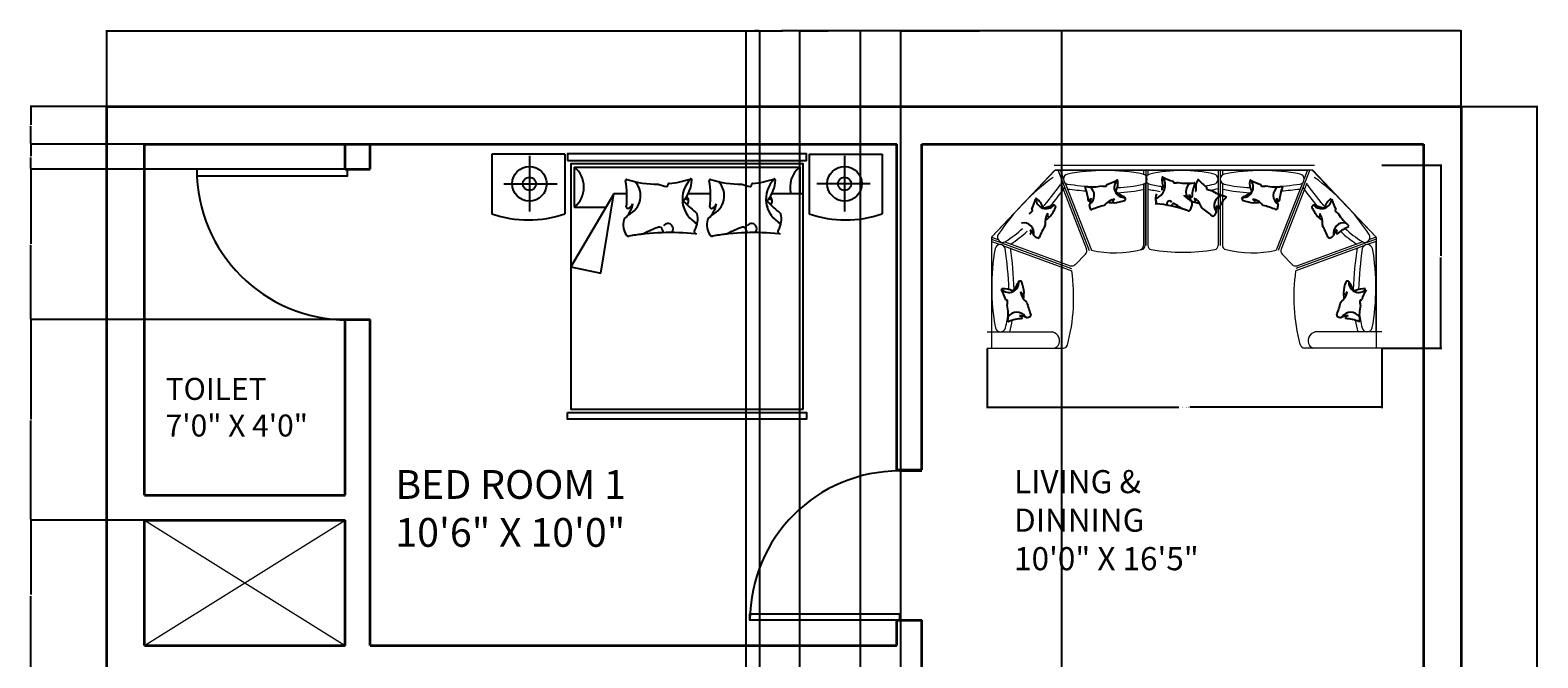
# Model space of a CAD drawing. Units: inches. Extents: x 2360 to 2721, y 1697 to 2094.
# Tile 3 of 3: x 2360 to 2721, y 1944 to 2094. Entities that reach past the tile are written whole.
import ezdxf

# ---------------------------------------------------------------- set-up
doc = ezdxf.new("R2010")
doc.units = ezdxf.units.IN
for name, color, linetype, lineweight in [('A-ANNO-DIMS', 2, 'Continuous', 18), ('A-AREA-IDEN', 7, 'Continuous', 18), ('A-DOOR', 4, 'Continuous', 25), ('A-FLOR-OPEN', 8, 'Continuous', 13), ('A-WALL', 7, 'Continuous', 35), ('FUR', 42, 'Continuous', 18)]:
    doc.layers.add(name, color=color, linetype=linetype, lineweight=lineweight)
for name, color, linetype in [('HID', 11, 'Continuous'), ('SAN', 5, 'Continuous'), ('wood', 26, 'Continuous')]:
    doc.layers.add(name, color=color, linetype=linetype)
doc.styles.get("Standard").update_dxf_attribs({"font": 'arial.ttf'})
doc.dimstyles.get("Standard").update_dxf_attribs({"dimtxt": 0.18, "dimasz": 0.18, "dimexe": 0.18, "dimexo": 0.0625, "dimgap": 0.09, "dimtad": 0, "dimtih": 1, "dimtoh": 1, "dimdec": 4, "dimzin": 0, "dimdsep": 46, "dimtxsty": 'Standard', "dimcen": 0.09, "dimadec": 0, "dimazin": 0, "dimtfac": 1, "dimtdec": 4, "dimtofl": 0, "dimtmove": 0, "dimatfit": 3, "dimfxl": 1, "dimtolj": 1, "dimtzin": 0, "dimarcsym": 0})

# ---------------------------------------------------------------- blocks, each defined once
blk = doc.blocks.new('*U2')
for p, q in [((0, 0), (0, -6)), ((-40, 0), (-40, -6))]:
    blk.add_line(p, q)
blk.add_lwpolyline([(0, 0), (0, 40), (-1.75, 40), (-1.75, 0)], close=True)
blk.add_arc((0, 0), 40, 90, 180)
blk = doc.blocks.new('*U3')
for p, q in [((0, 0), (0, -6)), ((40, 0), (40, -6))]:
    blk.add_line(p, q)
blk.add_lwpolyline([(0, 0), (0, 40), (1.75, 40), (1.75, 0)], close=True)
blk.add_arc((0, 0), 40, 0, 90)
blk = doc.blocks.new('A$C47AC156F')
at = {"layer": 'HID'}
for centre, radius, start, end in [((1.015, 1.799), 0.00933, 72.7248, 190.959), ((0.396, 1.679), 0.622, 352.7363, 10.959), ((1.25, 2.553), 0.781, 252.7248, 270.2702), ((0.966, 1.684), 0.155, 292.7628, 43.8922), ((1.385, 2.121), 0.373, 249.4168, 259.3085), ((1.317, 1.764), 0.00933, 259.3085, 10.689), ((1.336, 1.768), 0.00933, 96.2196, 190.689), ((1.25, 2.553), 0.781, 276.2196, 288.2114), ((1.645, 1.66), 0.21, 133.8947, 242.3952), ((1.258, 1.815), 0.249, 319.9211, 357.124), ((1.497, 1.803), 0.00933, 357.124, 108.2114), ((1.497, 1.803), 0.00933, 357.124, 108.2114), ((1.645, 1.799), 0.00933, 72.7248, 190.959), ((1.026, 1.679), 0.622, 352.7363, 10.959), ((1.88, 2.553), 0.781, 252.7248, 270.2702), ((1.596, 1.684), 0.155, 292.7628, 43.8922), ((2.015, 2.121), 0.373, 249.4168, 259.3085), ((1.947, 1.764), 0.00933, 259.3085, 10.689), ((1.966, 1.768), 0.00933, 96.2196, 190.689), ((1.88, 2.553), 0.781, 276.2196, 288.2114), ((2.275, 1.66), 0.21, 133.8947, 242.3952), ((1.888, 1.815), 0.249, 319.9211, 357.124), ((2.127, 1.803), 0.00933, 357.124, 108.2114), ((2.127, 1.803), 0.00933, 357.124, 108.2114), ((0.871, 1.658), 0.194, 311.6071, 349.7845), ((1.022, 1.599), 0.00933, 172.7363, 288.2985), ((1.005, 1.648), 0.0615, 288.2985, 335.7891), ((1.453, 1.646), 0.00933, 118.8315, 225.8329), ((2.727, 2.958), 1.838, 225.8329, 230.0245), ((0.994, -0.376), 2.088, 76.4982, 77.2888), ((0.994, 3.644), 2.088, 282.7018, 282.7206), ((1.445, 1.644), 0.0373, 312.662, 59.1573), ((1.501, 1.658), 0.194, 311.6071, 349.7845), ((1.652, 1.599), 0.00933, 172.7363, 288.2985), ((1.635, 1.648), 0.0615, 288.2985, 335.7891), ((2.083, 1.646), 0.00933, 118.8315, 225.8329), ((3.357, 2.958), 1.838, 225.8329, 230.0245), ((1.624, -0.376), 2.088, 76.4982, 77.2888), ((1.624, 3.644), 2.088, 282.7018, 282.7206), ((2.075, 1.644), 0.0373, 312.662, 59.1573), ((1.142, 1.469), 0.152, 167.3377, 211.666), ((1.012, 1.499), 0.0187, 131.6071, 167.3377), ((1.401, 1.508), 0.151, 327.1663, 15.7613), ((1.772, 1.469), 0.152, 167.3377, 211.666), ((1.642, 1.499), 0.0187, 131.6071, 167.3377), ((2.031, 1.508), 0.151, 327.1663, 15.7613), ((1.028, 1.399), 0.0187, 211.666, 279.4465), ((1.35, -0.534), 1.941, 84.5852, 99.4465), ((1.35, -0.534), 1.941, 96.386, 99.4465), ((1.132, 1.414), 0.0187, 276.386, 303.7955), ((1.54, 0.631), 0.864, 109.049, 117.3823), ((1.264, 1.43), 0.0187, 2.6426, 109.049), ((1.301, 1.432), 0.0187, 182.6426, 192.7015), ((1.323, 1.437), 0.0414, 192.7015, 227.1556), ((1.326, 1.436), 0.0395, 312.3565, 145.7762), ((1.543, 1.416), 0.0187, 147.1663, 264.3422), ((1.659, 1.399), 0.0187, 211.666, 279.4465), ((1.98, -0.534), 1.941, 84.5852, 99.4465), ((1.98, -0.534), 1.941, 96.386, 99.4465), ((1.762, 1.414), 0.0187, 276.386, 303.7955), ((2.17, 0.631), 0.864, 109.049, 117.3823), ((1.894, 1.43), 0.0187, 2.6426, 109.049), ((1.931, 1.432), 0.0187, 182.6426, 192.7015), ((1.954, 1.437), 0.0414, 192.7015, 227.1556), ((1.956, 1.436), 0.0395, 312.3565, 145.7762), ((2.173, 1.416), 0.0187, 147.1663, 264.3422)]:
    blk.add_arc(centre, radius, start, end, dxfattribs=at)
at = {"layer": 'SAN'}
for p, q in [((0.283, 1.985), (0.283, 1.566)), ((2.657, 1.985), (2.657, 1.566)), ((0.09, 1.775), (0.491, 1.775)), ((2.85, 1.775), (2.449, 1.775))]:
    blk.add_line(p, q, dxfattribs=at)
for centre, radius in [((0.283, 1.775), 0.13), ((0.283, 1.775), 0.05), ((2.657, 1.775), 0.13), ((2.657, 1.775), 0.05)]:
    blk.add_circle(centre, radius, dxfattribs=at)
at = {"layer": 'wood'}
for p, q in [((0, 1.998), (0, 1.548)), ((0.55, 1.998), (0, 1.998)), ((0.55, 1.998), (0.55, 1.548)), ((2.39, 1.998), (2.94, 1.998)), ((2.39, 1.998), (2.39, 1.548)), ((2.94, 1.998), (2.94, 1.548)), ((0.62, 1.9), (2.32, 1.9)), ((0.62, 1.9), (0.62, 1.6)), ((2.32, 1.9), (2.32, 1.7)), ((0.92, 1.7), (0.595, 1.15)), ((0.62, 1.6), (0.861, 1.6)), ((0.82, 1.1), (0.92, 1.7)), ((1.017, 1.7), (0.92, 1.7)), ((1.647, 1.7), (1.479, 1.7)), ((2.345, 1.7), (2.109, 1.7)), ((0.595, 1.15), (0.82, 1.1))]:
    blk.add_line(p, q, dxfattribs=at)
for points in [[(0.57, 1.95), (2.37, 1.95), (2.37, 2), (0.57, 2)], [(2.345, 0.075), (2.345, 1.925), (0.595, 1.925), (0.595, 0.075)], [(0.57, 0.05), (2.37, 0.05), (2.37, 0), (0.57, 0)]]:
    blk.add_lwpolyline(points, close=True, dxfattribs=at)
for centre, radius, start, end in [((0.504, 1.75), 0.19, 307.7826, 52.2174), ((2.436, 1.75), 0.19, 127.7826, 195.2747), ((0.275, 2.342), 0.84, 250.89, 289.11), ((2.665, 2.342), 0.84, 250.89, 289.11)]:
    blk.add_arc(centre, radius, start, end, dxfattribs=at)
blk = doc.blocks.new('A$C5B9B1B1E')
at = {"layer": 'FUR'}
for p, q in [((0.68, 1.857), (3.32, 1.857)), ((0.044, 1.127), (0.687, 1.804)), ((0.046, 1.126), (0.691, 1.805)), ((0.687, 1.804), (3.246, 1.804)), ((0.689, 1.807), (3.298, 1.807)), ((0.718, 1.807), (1.035, 0.991)), ((0.741, 1.807), (0.774, 1.719)), ((1.587, 1.804), (1.587, 1.757)), ((1.608, 1.804), (1.608, 1.041)), ((1.629, 1.804), (1.629, 1.757)), ((2.343, 1.804), (2.343, 1.041)), ((2.364, 1.804), (2.364, 1.041)), ((2.385, 1.804), (2.385, 1.757)), ((3.27, 1.807), (2.952, 0.991)), ((3.247, 1.807), (3.213, 1.719)), ((3.942, 1.126), (3.296, 1.805)), ((3.944, 1.127), (3.298, 1.807)), ((0.748, 1.672), (1.007, 1.005)), ((0.792, 1.675), (1.057, 0.993)), ((1.587, 1.671), (1.587, 1.041)), ((1.603, 1.671), (1.603, 1.041)), ((1.629, 1.671), (1.629, 1.041)), ((2.385, 1.671), (2.385, 1.041)), ((3.196, 1.675), (2.93, 0.993)), ((3.24, 1.672), (2.98, 1.005)), ((0.044, 1.127), (0.044, 0)), ((0.044, 1.127), (0.112, 1.103)), ((0.044, 1.105), (0.856, 0.808)), ((0.044, 1.083), (0.133, 1.05)), ((0.046, 1.082), (0.046, 0.164)), ((0.181, 1.077), (0.842, 0.836)), ((3.944, 1.105), (3.131, 0.808)), ((3.807, 1.077), (3.145, 0.836)), ((3.944, 1.083), (3.854, 1.05)), ((3.944, 1.127), (3.875, 1.103)), ((3.941, 1.082), (3.941, 0.164)), ((3.944, 1.127), (3.944, 0)), ((0.167, 1.038), (0.86, 0.785)), ((0.997, 0.952), (0.895, 0.848)), ((2.991, 0.952), (3.093, 0.848)), ((3.82, 1.038), (3.128, 0.785)), ((0, 0.164), (0.663, 0.164)), ((4, 0.164), (3.325, 0.164)), ((0, 0), (0.775, 0)), ((4, 0), (3.219, 0))]:
    blk.add_line(p, q, dxfattribs=at)
for centre, radius, start, end in [((1.999, -0.1), 2.263, 125.9311, 146.4201), ((0.827, 1.714), 0.0525, 104.0803, 255.9197), ((1.2, -0.267), 2.068, 79.3218, 100.7558), ((1.571, 1.714), 0.0529, 283.4421, 76.5579), ((1.661, 1.714), 0.0529, 103.4421, 256.5579), ((1.974, 0.302), 1.499, 77.3591, 102.5496), ((2.289, 1.714), 0.0525, 284.0803, 75.9197), ((2.417, 1.714), 0.0529, 103.4421, 256.5579), ((2.788, -0.267), 2.068, 79.2442, 100.6782), ((3.161, 1.714), 0.0525, 284.0803, 75.9197), ((1.989, -0.1), 2.263, 33.5799, 54.0689), ((-2.245, 3.806), 3.68, 319.5649, 324.3474), ((-2.245, 3.806), 3.733, 320.6889, 324.3474), ((1.373, 5.964), 4.337, 262.5873, 266.2564), ((1.493, 7.461), 5.886, 263.3874, 265.2569), ((1.257, 3.126), 1.499, 272.4014, 282.5496), ((1.257, 3.126), 1.551, 272.4014, 282.5496), ((1.974, 3.126), 1.551, 257.1404, 261.9048), ((1.974, 3.126), 1.499, 257.4504, 262.6454), ((1.974, 3.126), 1.499, 274.5548, 275.3997), ((1.974, 3.126), 1.499, 278.9885, 282.6409), ((1.974, 3.126), 1.551, 280.7847, 283.7486), ((2.73, 3.126), 1.551, 257.4504, 267.5986), ((2.73, 3.126), 1.499, 257.4504, 267.5986), ((2.614, 5.964), 4.337, 273.7436, 277.4127), ((2.494, 7.461), 5.886, 274.7431, 276.6126), ((6.233, 3.806), 3.733, 215.6526, 219.3111), ((6.233, 3.806), 3.68, 215.6526, 220.4351), ((0.159, 1.125), 0.0525, 149.9951, 301.8345), ((-0.635, 2.334), 1.499, 303.2739, 311.5982), ((-0.635, 2.334), 1.551, 304.4606, 312.1941), ((4.623, 2.334), 1.551, 227.8059, 235.5394), ((4.623, 2.334), 1.499, 228.4018, 236.7261), ((3.828, 1.125), 0.0525, 238.1655, 30.0049), ((2.31, 0.617), 2.263, 170.0163, 190.5053), ((0.133, 0.997), 0.0529, 13.4421, 166.5579), ((-3.456, 0.47), 3.68, 1.9572, 8.4326), ((-3.456, 0.47), 3.733, 1.9572, 8.4326), ((0.961, 0.987), 0.05, 315.6002, 21.264), ((1.299, 2.034), 1.068, 256.9274, 284.5801), ((1.545, 1.041), 0.042, 279.7794, 0), ((1.561, 1.041), 0.042, 279.7794, 0), ((1.671, 1.041), 0.042, 180, 260.2206), ((1.986, 2.869), 1.897, 260.2206, 279.7794), ((2.301, 1.041), 0.042, 279.7794, 0), ((2.427, 1.041), 0.042, 180, 260.2206), ((2.689, 2.034), 1.068, 255.4199, 283.0726), ((3.027, 0.987), 0.05, 158.736, 224.3998), ((7.443, 0.47), 3.733, 171.5674, 178.0428), ((7.443, 0.47), 3.68, 171.5674, 178.0428), ((3.854, 0.997), 0.0529, 13.4421, 166.5579), ((1.678, 0.617), 2.263, 349.4947, 9.9837), ((-1.061, 0.519), 1.939, 345.4239, 7.8665), ((0.859, 0.883), 0.05, 249.9365, 315.6002), ((3.128, 0.883), 0.05, 224.3998, 290.0635), ((5.006, 0.521), 1.897, 172.0077, 194.7607), ((-1.275, 0.533), 1.499, 347.3591, 353.601), ((5.263, 0.533), 1.499, 186.399, 192.6409), ((0.136, 0.218), 0.0525, 194.0803, 345.9197), ((-1.275, 0.533), 1.551, 346.2514, 350.7022), ((0.643, 0.074), 0.0918, 328.6411, 77.5888), ((3.345, 0.074), 0.0918, 102.4112, 211.3589), ((5.263, 0.533), 1.551, 189.2978, 193.7486), ((3.851, 0.218), 0.0525, 194.0803, 345.9197), ((0.665, 0.069), 0.0703, 279.5212, 322.6757), ((0.775, 0.042), 0.042, 270, 345.2393), ((3.226, 0.057), 0.0573, 199.356, 262.7582), ((3.338, 0.086), 0.0936, 219.4969, 247.1448)]:
    blk.add_arc(centre, radius, start, end, dxfattribs=at)
at = {"layer": 'HID'}
for centre, radius, start, end in [((1.056, 2.162), 0.527, 287.478, 299.4698), ((1.393, 1.632), 0.104, 135.6927, 273.5175), ((1.159, 1.674), 0.168, 330.4242, 8.3824), ((1.319, 1.698), 0.0063, 8.3824, 119.4698), ((1.664, 1.652), 0.142, 287.6048, 36.1053), ((1.94, 1.709), 0.168, 172.876, 210.0789), ((1.78, 1.729), 0.0063, 61.7886, 172.876), ((1.78, 1.729), 0.0063, 61.7886, 172.876), ((2.032, 2.199), 0.527, 241.7886, 253.7804), ((1.883, 1.687), 0.0063, 339.311, 73.7804), ((1.895, 1.683), 0.0063, 159.311, 270.6915), ((2.283, 1.626), 0.168, 151.6176, 189.5758), ((2.141, 1.703), 0.0063, 40.5302, 151.6176), ((2.546, 2.05), 0.527, 220.5302, 232.522), ((2.594, 1.632), 0.104, 266.4825, 44.3073), ((2.829, 1.674), 0.168, 171.6176, 209.5758), ((2.669, 1.698), 0.0063, 60.5302, 171.6176), ((2.931, 2.162), 0.527, 240.5302, 252.522), ((1, 1.632), 0.0063, 83.9832, 202.2174), ((0.606, 1.471), 0.42, 3.9947, 22.2174), ((1.056, 2.162), 0.527, 263.9832, 281.5286), ((0.982, 1.549), 0.105, 304.0212, 55.1506), ((1.202, 1.894), 0.252, 260.6752, 270.5669), ((1.205, 1.649), 0.0063, 270.5669, 21.9475), ((1.216, 1.653), 0.0063, 107.478, 201.9475), ((1.31, 1.588), 0.0063, 150.4242, 237.1103), ((1.981, 2.625), 1.241, 237.1103, 241.1368), ((1.379, 1.514), 0.0244, 343.8009, 85.0524), ((1.809, 1.522), 0.102, 154.2387, 202.8337), ((1.795, 1.618), 0.0252, 110.8427, 217.338), ((1.859, 0.222), 1.409, 92.7112, 93.5018), ((2.33, 2.894), 1.409, 247.2794, 247.2982), ((1.791, 1.62), 0.0063, 304.1671, 51.1685), ((1.892, 1.928), 0.252, 270.6915, 280.5832), ((2.032, 2.199), 0.527, 259.7298, 277.2752), ((2.009, 1.552), 0.0126, 176.1991, 230.6607), ((2.302, 1.91), 0.476, 230.6607, 243.8744), ((2.119, 1.588), 0.105, 126.1078, 237.2372), ((2.088, 1.569), 0.0416, 194.2109, 241.7015), ((2.179, 1.559), 0.131, 180.2155, 218.3929), ((2.072, 1.538), 0.0063, 241.7015, 357.2637), ((2.497, 1.518), 0.42, 159.041, 177.2637), ((2.099, 1.67), 0.0063, 339.041, 97.2752), ((2.111, 1.597), 0.0063, 282.8897, 9.5758), ((2.231, 1.618), 0.0063, 138.0525, 249.4331), ((2.222, 1.627), 0.0063, 318.0525, 52.522), ((2.317, 1.848), 0.252, 249.4331, 259.3248), ((2.546, 2.05), 0.527, 238.4714, 256.0168), ((2.406, 1.449), 0.105, 104.8494, 215.9788), ((2.417, 1.532), 0.0063, 317.7826, 76.0168), ((2.608, 1.514), 0.0244, 94.9476, 196.1991), ((2.007, 2.625), 1.241, 298.8632, 302.8897), ((2.677, 1.588), 0.0063, 302.8897, 29.5758), ((2.771, 1.653), 0.0063, 338.0525, 72.522), ((2.783, 1.649), 0.0063, 158.0525, 269.4331), ((2.785, 1.894), 0.252, 269.4331, 279.3248), ((2.931, 2.162), 0.527, 258.4714, 276.0168), ((3.005, 1.549), 0.105, 124.8494, 235.9788), ((3.382, 1.471), 0.42, 157.7826, 176.0053), ((2.987, 1.632), 0.0063, 337.7826, 96.0168), ((0.277, 1.564), 0.252, 306.59, 316.4817), ((0.459, 1.407), 0.0063, 153.3928, 247.8623), ((-0.018, 1.646), 0.527, 333.3928, 345.3846), ((0.455, 1.395), 0.0063, 316.4817, 67.8623), ((0.498, 1.511), 0.0063, 54.2972, 165.3846), ((0.598, 1.519), 0.104, 181.6075, 319.4323), ((0.404, 1.38), 0.168, 16.339, 54.2972), ((0.571, 1.429), 0.0063, 196.339, 283.0251), ((0.293, 2.632), 1.241, 283.0251, 287.0516), ((0.263, 1.627), 0.476, 322.0404, 335.2541), ((0.673, 1.427), 0.0244, 29.7157, 130.9672), ((0.683, 1.433), 0.0126, 335.2541, 29.7157), ((1.031, 1.5), 0.0063, 183.9947, 299.557), ((1.013, 1.531), 0.0416, 299.557, 347.0475), ((0.923, 1.519), 0.131, 329.5087, 1.0429), ((1.135, 1.458), 0.099, 182.7962, 207.1304), ((1.058, 1.418), 0.0126, 207.1304, 290.9482), ((1.531, 0.183), 1.31, 105.1521, 110.9482), ((1.185, 1.46), 0.0126, 285.1521, 322.4345), ((1.324, 1.352), 0.163, 100.921, 142.4345), ((1.274, 1.728), 0.252, 258.5381, 270.9308), ((1.286, 1.487), 0.0126, 131.4659, 280.4525), ((1.185, 1.602), 0.141, 311.4659, 320.8131), ((1.237, 1.948), 0.476, 276.1256, 289.3393), ((1.391, 1.511), 0.0126, 289.3393, 343.8009), ((1.704, 1.478), 0.0126, 265.6578, 22.8337), ((1.603, 0.159), 1.31, 70.5535, 85.4148), ((1.85, 1.466), 0.0267, 24.2238, 217.6435), ((1.852, 1.466), 0.0279, 302.8444, 337.2985), ((1.866, 1.46), 0.0126, 337.2985, 347.3574), ((1.891, 1.454), 0.0126, 60.951, 167.3574), ((1.614, 0.955), 0.583, 52.6177, 60.951), ((1.977, 1.428), 0.0126, 226.2045, 253.614), ((1.603, 0.159), 1.31, 70.5535, 73.614), ((2.044, 1.406), 0.0126, 250.5535, 318.334), ((1.976, 1.466), 0.103, 318.334, 2.6623), ((2.067, 1.47), 0.0126, 2.6623, 38.3929), ((2.099, 1.494), 0.0126, 239.5475, 28.5341), ((2.234, 1.567), 0.141, 199.1869, 208.5341), ((2.017, 1.381), 0.163, 17.5655, 59.079), ((2.193, 1.717), 0.252, 249.0692, 261.4619), ((2.185, 1.434), 0.0126, 197.5655, 234.8479), ((1.423, 0.352), 1.31, 49.0518, 54.8479), ((2.232, 1.415), 0.099, 312.8696, 337.2038), ((2.452, 1.4), 0.131, 158.9571, 190.4913), ((2.371, 1.442), 0.0416, 172.9525, 220.443), ((2.344, 1.419), 0.0063, 220.443, 336.0053), ((2.733, 1.246), 0.42, 137.7826, 156.0053), ((2.597, 1.511), 0.0126, 196.1991, 250.6607), ((2.75, 1.948), 0.476, 250.6607, 263.8744), ((2.663, 1.352), 0.163, 37.5655, 79.079), ((2.803, 1.602), 0.141, 219.1869, 228.5341), ((2.702, 1.487), 0.0126, 259.5475, 48.5341), ((2.713, 1.728), 0.252, 269.0692, 281.4619), ((2.803, 1.46), 0.0126, 217.5655, 254.8479), ((2.457, 0.183), 1.31, 69.0518, 74.8479), ((2.93, 1.418), 0.0126, 249.0518, 332.8696), ((3.065, 1.519), 0.131, 178.9571, 210.4913), ((2.974, 1.531), 0.0416, 192.9525, 240.443), ((2.853, 1.458), 0.099, 332.8696, 357.2038), ((2.957, 1.5), 0.0063, 240.443, 356.0053), ((3.304, 1.433), 0.0126, 150.2843, 204.7459), ((3.315, 1.427), 0.0244, 49.0328, 150.2843), ((3.725, 1.627), 0.476, 204.7459, 217.9596), ((3.389, 1.519), 0.104, 220.5677, 358.3925), ((3.694, 2.632), 1.241, 252.9484, 256.9749), ((3.416, 1.429), 0.0063, 256.9749, 343.661), ((3.583, 1.38), 0.168, 125.7028, 163.661), ((4.005, 1.646), 0.527, 194.6154, 206.6072), ((3.533, 1.395), 0.0063, 112.1377, 223.5183), ((3.711, 1.564), 0.252, 223.5183, 233.41), ((3.528, 1.407), 0.0063, 292.1377, 26.6072), ((0.371, 1.166), 0.105, 349.936, 101.0654), ((1.734, 0.609), 1.31, 151.0669, 156.863), ((0.751, 1.275), 0.163, 146.8358, 188.3493), ((0.446, 1.501), 0.252, 304.4529, 316.8456), ((0.577, 1.249), 0.0126, 331.0669, 8.3493), ((0.474, 1.348), 0.141, 357.3807, 6.7279), ((0.627, 1.341), 0.0126, 177.3807, 326.3673), ((2.29, 1.351), 0.0126, 229.0518, 312.8696), ((3.36, 1.341), 0.0126, 213.6327, 2.6193), ((3.542, 1.501), 0.252, 223.1544, 235.5471), ((3.513, 1.348), 0.141, 173.2721, 182.6193), ((3.237, 1.275), 0.163, 351.6507, 33.1642), ((3.411, 1.249), 0.0126, 171.6507, 208.9331), ((2.253, 0.609), 1.31, 23.137, 28.9331), ((3.616, 1.166), 0.105, 78.9346, 190.064), ((3.822, 0.841), 0.42, 111.8678, 130.0905), ((4.005, 1.646), 0.527, 212.5566, 230.102), ((0.44, 1.167), 0.0063, 229.9095, 345.4718), ((0.406, 1.176), 0.0416, 345.4718, 32.9623), ((0.351, 1.103), 0.131, 15.4235, 46.9577), ((0.543, 1.212), 0.099, 228.711, 253.0452), ((0.518, 1.129), 0.0126, 253.0452, 336.863), ((3.47, 1.129), 0.0126, 203.137, 286.9548), ((3.445, 1.212), 0.099, 286.9548, 311.289), ((3.636, 1.103), 0.131, 133.0423, 164.5765), ((3.582, 1.176), 0.0416, 147.0377, 194.5282), ((3.547, 1.167), 0.0063, 194.5282, 310.0905), ((0.219, 0.669), 0.104, 225.6927, 3.5175), ((-0.775, 1.256), 1.241, 327.1103, 331.1368), ((0.336, 0.655), 0.0244, 73.8009, 175.0524), ((0.34, 0.666), 0.0126, 19.3393, 73.8009), ((-0.097, 0.513), 0.476, 6.1256, 19.3393), ((4.085, 0.513), 0.476, 160.6607, 173.8744), ((3.648, 0.666), 0.0126, 106.1991, 160.6607), ((3.651, 0.655), 0.0244, 4.9476, 106.1991), ((3.769, 0.669), 0.104, 176.4825, 314.3073), ((4.762, 1.256), 1.241, 208.8632, 212.8897), ((0.152, 0.594), 0.0063, 98.3824, 209.4698), ((-0.312, 0.331), 0.527, 17.478, 29.4698), ((0.176, 0.434), 0.168, 60.4242, 98.3824), ((0.197, 0.492), 0.0063, 197.478, 291.9475), ((0.202, 0.48), 0.0063, 0.5669, 111.9475), ((-0.044, 0.478), 0.252, 350.6752, 0.5669), ((0.262, 0.586), 0.0063, 240.4242, 327.1103), ((0.498, 0.6), 0.163, 190.921, 232.4345), ((0.249, 0.46), 0.141, 41.4659, 50.8131), ((0.363, 0.561), 0.0126, 221.4659, 10.4525), ((0.122, 0.55), 0.252, 348.5381, 0.9308), ((0.391, 0.46), 0.0126, 15.1521, 52.4345), ((1.668, 0.806), 1.31, 195.1521, 200.9482), ((2.32, 0.806), 1.31, 339.0518, 344.8479), ((3.597, 0.46), 0.0126, 127.5655, 164.8479), ((3.49, 0.6), 0.163, 307.5655, 349.079), ((3.624, 0.561), 0.0126, 169.5475, 318.5341), ((3.866, 0.55), 0.252, 179.0692, 191.4619), ((3.739, 0.46), 0.141, 129.1869, 138.5341), ((3.726, 0.586), 0.0063, 212.8897, 299.5758), ((3.811, 0.434), 0.168, 81.6176, 119.5758), ((3.786, 0.48), 0.0063, 68.0525, 179.4331), ((4.031, 0.478), 0.252, 179.4331, 189.3248), ((3.791, 0.492), 0.0063, 248.0525, 342.522), ((4.3, 0.331), 0.527, 150.5302, 162.522), ((-0.312, 0.331), 0.527, 353.9832, 11.5286), ((0.301, 0.258), 0.105, 34.0212, 145.1506), ((0.319, 0.289), 0.0416, 29.557, 77.0475), ((0.331, 0.198), 0.131, 59.5087, 91.0429), ((0.35, 0.306), 0.0063, 273.9947, 29.557), ((0.393, 0.41), 0.099, 272.7962, 297.1304), ((0.432, 0.333), 0.0126, 297.1304, 20.9482), ((3.556, 0.333), 0.0126, 159.0518, 242.8696), ((3.595, 0.41), 0.099, 242.8696, 267.2038), ((3.657, 0.198), 0.131, 88.9571, 120.4913), ((3.687, 0.258), 0.105, 34.8494, 145.9788), ((3.638, 0.306), 0.0063, 150.443, 266.0053), ((3.668, 0.289), 0.0416, 102.9525, 150.443), ((4.3, 0.331), 0.527, 168.4714, 186.0168), ((0.219, 0.276), 0.0063, 173.9832, 292.2174), ((0.38, -0.119), 0.42, 93.9947, 112.2174), ((3.608, -0.119), 0.42, 67.7826, 86.0053), ((3.769, 0.276), 0.0063, 247.7826, 6.0168)]:
    blk.add_arc(centre, radius, start, end, dxfattribs=at)
blk = doc.blocks.new('*D11')
at = {"layer": 'A-ANNO-DIMS', "color": 0, "lineweight": -2, "transparency": 16777216}
for p, q in [((2589.22, 2017.76), (2589.22, 2003.48)), ((2683.64, 2017.76), (2683.64, 2003.48)), ((2589.4, 2003.66), (2635.09, 2003.66)), ((2683.46, 2003.66), (2637.77, 2003.66))]:
    blk.add_line(p, q, dxfattribs=at)
at = {"layer": 'A-ANNO-DIMS', "color": 0, "transparency": 16777216}
for points in [[(2589.4, 2003.69), (2589.4, 2003.63), (2589.22, 2003.66)], [(2683.46, 2003.69), (2683.46, 2003.63), (2683.64, 2003.66)]]:
    blk.add_solid(points, dxfattribs=at)
at = {"layer": 'Defpoints', "color": 0, "transparency": 16777216}
for p in [(2589.22, 2017.83), (2683.64, 2017.83), (2683.64, 2003.66)]:
    blk.add_point(p, dxfattribs=at)
at = {"layer": 'A-ANNO-DIMS', "color": 0, "transparency": 16777216, "insert": (2636.43, 2003.66), "char_height": 0.18, "attachment_point": 5}
blk.add_mtext('\\A1;SECTIONAL SOFA 94', dxfattribs=at)
blk = doc.blocks.new('*D12')
at = {"layer": 'A-ANNO-DIMS', "color": 0, "lineweight": -2, "transparency": 16777216}
for p, q in [((2683.7, 2061.65), (2697.98, 2061.65)), ((2697.8, 2061.47), (2697.8, 2039.92)), ((2697.8, 2018.01), (2697.8, 2039.56)), ((2683.7, 2017.83), (2697.98, 2017.83))]:
    blk.add_line(p, q, dxfattribs=at)
at = {"layer": 'A-ANNO-DIMS', "color": 0, "transparency": 16777216}
for points in [[(2697.77, 2061.47), (2697.83, 2061.47), (2697.8, 2061.65)], [(2697.77, 2018.01), (2697.83, 2018.01), (2697.8, 2017.83)]]:
    blk.add_solid(points, dxfattribs=at)
at = {"layer": 'Defpoints', "color": 0, "transparency": 16777216}
for p in [(2683.64, 2061.65), (2697.8, 2061.65), (2683.64, 2017.83)]:
    blk.add_point(p, dxfattribs=at)
at = {"layer": 'A-ANNO-DIMS', "color": 0, "transparency": 16777216, "insert": (2697.8, 2039.74), "char_height": 0.18, "attachment_point": 5}
blk.add_mtext('\\A1;44', dxfattribs=at)
blk = doc.blocks.new('*D17')
at = {"layer": 'A-ANNO-DIMS', "color": 0, "lineweight": -2, "transparency": 16777216}
for p, q in [((2378.63, 2075.71), (2378.63, 2093.98)), ((2378.81, 2093.8), (2540.34, 2093.8)), ((2702.45, 2093.8), (2540.92, 2093.8)), ((2702.63, 2075.71), (2702.63, 2093.98))]:
    blk.add_line(p, q, dxfattribs=at)
at = {"layer": 'A-ANNO-DIMS', "color": 0, "transparency": 16777216}
for points in [[(2378.81, 2093.83), (2378.81, 2093.77), (2378.63, 2093.8)], [(2702.45, 2093.83), (2702.45, 2093.77), (2702.63, 2093.8)]]:
    blk.add_solid(points, dxfattribs=at)
at = {"layer": 'Defpoints', "color": 0, "transparency": 16777216}
for p in [(2702.63, 2093.8), (2378.63, 2075.65), (2702.63, 2075.65)]:
    blk.add_point(p, dxfattribs=at)
at = {"layer": 'A-ANNO-DIMS', "color": 0, "transparency": 16777216, "insert": (2540.63, 2093.8), "char_height": 0.18, "attachment_point": 5}
blk.add_mtext('\\A1;324', dxfattribs=at)
blk = doc.blocks.new('*D18')
at = {"layer": 'A-ANNO-DIMS', "color": 0, "lineweight": -2, "transparency": 16777216}
for p, q in [((2702.69, 2075.65), (2720.96, 2075.65)), ((2720.78, 2075.47), (2720.78, 1895.83)), ((2720.78, 1715.83), (2720.78, 1895.46)), ((2702.69, 1715.65), (2720.96, 1715.65))]:
    blk.add_line(p, q, dxfattribs=at)
at = {"layer": 'A-ANNO-DIMS', "color": 0, "transparency": 16777216}
for points in [[(2720.75, 2075.47), (2720.81, 2075.47), (2720.78, 2075.65)], [(2720.75, 1715.83), (2720.81, 1715.83), (2720.78, 1715.65)]]:
    blk.add_solid(points, dxfattribs=at)
at = {"layer": 'Defpoints', "color": 0, "transparency": 16777216}
for p in [(2702.63, 2075.65), (2720.78, 2075.65), (2702.63, 1715.65)]:
    blk.add_point(p, dxfattribs=at)
at = {"layer": 'A-ANNO-DIMS', "color": 0, "transparency": 16777216, "insert": (2720.78, 1895.65), "char_height": 0.18, "attachment_point": 5}
blk.add_mtext('\\A1;360', dxfattribs=at)
blk = doc.blocks.new('*D26')
at = {"layer": 'A-ANNO-DIMS', "color": 0, "lineweight": -2, "transparency": 16777216}
for p, q in [((2387.57, 1976.65), (2360.3, 1976.65)), ((2360.48, 1976.47), (2360.48, 1958.83)), ((2360.48, 1940.83), (2360.48, 1958.46)), ((2387.57, 1940.65), (2360.3, 1940.65))]:
    blk.add_line(p, q, dxfattribs=at)
at = {"layer": 'A-ANNO-DIMS', "color": 0, "transparency": 16777216}
for points in [[(2360.45, 1976.47), (2360.51, 1976.47), (2360.48, 1976.65)], [(2360.45, 1940.83), (2360.51, 1940.83), (2360.48, 1940.65)]]:
    blk.add_solid(points, dxfattribs=at)
at = {"layer": 'Defpoints', "color": 0, "transparency": 16777216}
for p in [(2360.48, 1976.65), (2387.63, 1976.65), (2387.63, 1940.65)]:
    blk.add_point(p, dxfattribs=at)
at = {"layer": 'A-ANNO-DIMS', "color": 0, "transparency": 16777216, "insert": (2360.48, 1958.65), "char_height": 0.18, "attachment_point": 5}
blk.add_mtext('\\A1;36', dxfattribs=at)
blk = doc.blocks.new('*D27')
at = {"layer": 'A-ANNO-DIMS', "color": 0, "lineweight": -2, "transparency": 16777216}
for p, q in [((2435.57, 2024.65), (2360.3, 2024.65)), ((2360.48, 2024.47), (2360.48, 2000.83)), ((2360.48, 1976.83), (2360.48, 2000.46)), ((2387.57, 1976.65), (2360.3, 1976.65))]:
    blk.add_line(p, q, dxfattribs=at)
at = {"layer": 'A-ANNO-DIMS', "color": 0, "transparency": 16777216}
for points in [[(2360.45, 2024.47), (2360.51, 2024.47), (2360.48, 2024.65)], [(2360.45, 1976.83), (2360.51, 1976.83), (2360.48, 1976.65)]]:
    blk.add_solid(points, dxfattribs=at)
at = {"layer": 'Defpoints', "color": 0, "transparency": 16777216}
for p in [(2360.48, 2024.65), (2435.63, 2024.65), (2387.63, 1976.65)]:
    blk.add_point(p, dxfattribs=at)
at = {"layer": 'A-ANNO-DIMS', "color": 0, "transparency": 16777216, "insert": (2360.48, 2000.65), "char_height": 0.18, "attachment_point": 5}
blk.add_mtext('\\A1;48', dxfattribs=at)
blk = doc.blocks.new('*D28')
at = {"layer": 'A-ANNO-DIMS', "color": 0, "lineweight": -2, "transparency": 16777216}
for p, q in [((2435.57, 2060.65), (2360.3, 2060.65)), ((2360.48, 2060.47), (2360.48, 2042.83)), ((2360.48, 2024.83), (2360.48, 2042.46)), ((2435.57, 2024.65), (2360.3, 2024.65))]:
    blk.add_line(p, q, dxfattribs=at)
at = {"layer": 'A-ANNO-DIMS', "color": 0, "transparency": 16777216}
for points in [[(2360.45, 2060.47), (2360.51, 2060.47), (2360.48, 2060.65)], [(2360.45, 2024.83), (2360.51, 2024.83), (2360.48, 2024.65)]]:
    blk.add_solid(points, dxfattribs=at)
at = {"layer": 'Defpoints', "color": 0, "transparency": 16777216}
for p in [(2360.48, 2060.65), (2435.63, 2060.65), (2435.63, 2024.65)]:
    blk.add_point(p, dxfattribs=at)
at = {"layer": 'A-ANNO-DIMS', "color": 0, "transparency": 16777216, "insert": (2360.48, 2042.65), "char_height": 0.18, "attachment_point": 5}
blk.add_mtext('\\A1;36', dxfattribs=at)
blk = doc.blocks.new('*D29')
at = {"layer": 'A-ANNO-DIMS', "color": 0, "lineweight": -2, "transparency": 16777216}
for p, q in [((2435.57, 2066.65), (2360.3, 2066.65)), ((2360.48, 2066.47), (2360.48, 2063.83)), ((2360.48, 2060.83), (2360.48, 2063.46)), ((2435.57, 2060.65), (2360.3, 2060.65))]:
    blk.add_line(p, q, dxfattribs=at)
at = {"layer": 'A-ANNO-DIMS', "color": 0, "transparency": 16777216}
for points in [[(2360.45, 2066.47), (2360.51, 2066.47), (2360.48, 2066.65)], [(2360.45, 2060.83), (2360.51, 2060.83), (2360.48, 2060.65)]]:
    blk.add_solid(points, dxfattribs=at)
at = {"layer": 'Defpoints', "color": 0, "transparency": 16777216}
for p in [(2360.48, 2066.65), (2435.63, 2066.65), (2435.63, 2060.65)]:
    blk.add_point(p, dxfattribs=at)
at = {"layer": 'A-ANNO-DIMS', "color": 0, "transparency": 16777216, "insert": (2360.48, 2063.65), "char_height": 0.18, "attachment_point": 5}
blk.add_mtext('\\A1;6', dxfattribs=at)
blk = doc.blocks.new('*D30')
at = {"layer": 'A-ANNO-DIMS', "color": 0, "lineweight": -2, "transparency": 16777216}
for p, q in [((2378.57, 2075.65), (2360.3, 2075.65)), ((2360.48, 2075.47), (2360.48, 2071.33)), ((2360.48, 2066.83), (2360.48, 2070.96)), ((2387.57, 2066.65), (2360.3, 2066.65))]:
    blk.add_line(p, q, dxfattribs=at)
at = {"layer": 'A-ANNO-DIMS', "color": 0, "transparency": 16777216}
for points in [[(2360.45, 2075.47), (2360.51, 2075.47), (2360.48, 2075.65)], [(2360.45, 2066.83), (2360.51, 2066.83), (2360.48, 2066.65)]]:
    blk.add_solid(points, dxfattribs=at)
at = {"layer": 'Defpoints', "color": 0, "transparency": 16777216}
for p in [(2360.48, 2075.65), (2378.63, 2075.65), (2387.63, 2066.65)]:
    blk.add_point(p, dxfattribs=at)
at = {"layer": 'A-ANNO-DIMS', "color": 0, "transparency": 16777216, "insert": (2360.48, 2071.15), "char_height": 0.18, "attachment_point": 5}
blk.add_mtext('\\A1;9', dxfattribs=at)
blk = doc.blocks.new('*D33')
at = {"layer": 'A-ANNO-DIMS', "color": 0, "lineweight": -2, "transparency": 16777216}
for p, q in [((2568.56, 1756.6), (2568.56, 2093.98)), ((2568.74, 2093.8), (2587.43, 2093.8)), ((2606.92, 2093.8), (2588.22, 2093.8)), ((2607.1, 1756.6), (2607.1, 2093.98))]:
    blk.add_line(p, q, dxfattribs=at)
at = {"layer": 'A-ANNO-DIMS', "color": 0, "transparency": 16777216}
for points in [[(2568.74, 2093.83), (2568.74, 2093.77), (2568.56, 2093.8)], [(2606.92, 2093.83), (2606.92, 2093.77), (2607.1, 2093.8)]]:
    blk.add_solid(points, dxfattribs=at)
at = {"layer": 'Defpoints', "color": 0, "transparency": 16777216}
for p in [(2607.1, 2093.8), (2568.56, 1756.53), (2607.1, 1756.53)]:
    blk.add_point(p, dxfattribs=at)
at = {"layer": 'A-ANNO-DIMS', "color": 0, "transparency": 16777216, "insert": (2587.83, 2093.8), "char_height": 0.18, "attachment_point": 5}
blk.add_mtext('\\A1;38.54', dxfattribs=at)
blk = doc.blocks.new('*D34')
at = {"layer": 'A-ANNO-DIMS', "color": 0, "lineweight": -2, "transparency": 16777216}
for p, q in [((2544.47, 1742.14), (2544.47, 2093.98)), ((2544.65, 2093.8), (2551.24, 2093.8)), ((2558.74, 2093.8), (2552.15, 2093.8)), ((2558.92, 1742.14), (2558.92, 2093.98))]:
    blk.add_line(p, q, dxfattribs=at)
at = {"layer": 'A-ANNO-DIMS', "color": 0, "transparency": 16777216}
for points in [[(2544.65, 2093.83), (2544.65, 2093.77), (2544.47, 2093.8)], [(2558.74, 2093.83), (2558.74, 2093.77), (2558.92, 2093.8)]]:
    blk.add_solid(points, dxfattribs=at)
at = {"layer": 'Defpoints', "color": 0, "transparency": 16777216}
for p in [(2558.92, 2093.8), (2544.47, 1742.08), (2558.92, 1742.08)]:
    blk.add_point(p, dxfattribs=at)
at = {"layer": 'A-ANNO-DIMS', "color": 0, "transparency": 16777216, "insert": (2551.69, 2093.8), "char_height": 0.18, "attachment_point": 5}
blk.add_mtext('\\A1;14.454', dxfattribs=at)
blk = doc.blocks.new('*D35')
at = {"layer": 'A-ANNO-DIMS', "color": 0, "lineweight": -2, "transparency": 16777216}
for p, q in [((2534.83, 1727.69), (2534.83, 2093.98)), ((2535.01, 2093.8), (2539.25, 2093.8)), ((2544.29, 2093.8), (2540.04, 2093.8)), ((2544.47, 1742.14), (2544.47, 2093.98))]:
    blk.add_line(p, q, dxfattribs=at)
at = {"layer": 'A-ANNO-DIMS', "color": 0, "transparency": 16777216}
for points in [[(2535.01, 2093.83), (2535.01, 2093.77), (2534.83, 2093.8)], [(2544.29, 2093.83), (2544.29, 2093.77), (2544.47, 2093.8)]]:
    blk.add_solid(points, dxfattribs=at)
at = {"layer": 'Defpoints', "color": 0, "transparency": 16777216}
for p in [(2544.47, 2093.8), (2544.47, 1742.08), (2534.83, 1727.63)]:
    blk.add_point(p, dxfattribs=at)
at = {"layer": 'A-ANNO-DIMS', "color": 0, "transparency": 16777216, "insert": (2539.65, 2093.8), "char_height": 0.18, "attachment_point": 5}
blk.add_mtext('\\A1;9.636', dxfattribs=at)
blk = doc.blocks.new('*D37')
at = {"layer": 'A-ANNO-DIMS', "color": 0, "lineweight": -2, "transparency": 16777216}
for p, q in [((2531.63, 1724.71), (2531.63, 2093.98)), ((2531.81, 2093.8), (2532.84, 2093.8)), ((2534.65, 2093.8), (2533.63, 2093.8)), ((2534.83, 1727.69), (2534.83, 2093.98))]:
    blk.add_line(p, q, dxfattribs=at)
at = {"layer": 'A-ANNO-DIMS', "color": 0, "transparency": 16777216}
for points in [[(2531.81, 2093.83), (2531.81, 2093.77), (2531.63, 2093.8)], [(2534.65, 2093.83), (2534.65, 2093.77), (2534.83, 2093.8)]]:
    blk.add_solid(points, dxfattribs=at)
at = {"layer": 'Defpoints', "color": 0, "transparency": 16777216}
for p in [(2534.83, 2093.8), (2531.63, 1724.65), (2534.83, 1727.63)]:
    blk.add_point(p, dxfattribs=at)
at = {"layer": 'A-ANNO-DIMS', "color": 0, "transparency": 16777216, "insert": (2533.23, 2093.8), "char_height": 0.18, "attachment_point": 5}
blk.add_mtext('\\A1;3.198', dxfattribs=at)

msp = doc.modelspace()

# ---------------------------------------------------------------- linework, layer by layer
at = {"layer": 'A-FLOR-OPEN'}
for p, q in [((2387.6324, 1946.6468), (2435.6324, 1976.6468)), ((2387.6324, 1976.6468), (2435.6324, 1946.6468))]:
    msp.add_line(p, q, dxfattribs=at)
at = {"layer": 'A-WALL'}
for p, q in [((2378.6324, 2075.6468), (2702.6324, 2075.6468)), ((2378.6324, 1715.6468), (2378.6324, 2075.6468)), ((2702.6324, 2075.6468), (2702.6324, 1735.5718)), ((2387.6324, 2066.6468), (2567.6324, 2066.6468)), ((2387.6324, 1982.6468), (2387.6324, 2066.6468)), ((2435.6324, 2060.6468), (2435.6324, 2066.6468)), ((2441.6324, 2060.6468), (2441.6324, 2066.6468)), ((2567.6324, 1988.6468), (2567.6324, 2066.6468)), ((2573.6324, 1988.6468), (2573.6324, 2066.6468)), ((2573.6324, 2066.6468), (2693.6324, 2066.6468)), ((2693.6324, 2066.6468), (2693.6324, 1868.6468)), ((2435.6324, 2060.6468), (2441.6324, 2060.6468)), ((2435.6324, 2024.6468), (2441.6324, 2024.6468)), ((2435.6324, 1982.6468), (2435.6324, 2024.6468)), ((2441.6324, 1946.6468), (2441.6324, 2024.6468)), ((2567.6324, 1988.6468), (2573.6324, 1988.6468)), ((2387.6324, 1982.6468), (2435.6324, 1982.6468)), ((2387.6324, 1976.6468), (2435.6324, 1976.6468)), ((2387.6324, 1946.6468), (2387.6324, 1976.6468)), ((2435.6324, 1946.6468), (2435.6324, 1976.6468)), ((2567.6324, 1946.6468), (2567.6324, 1952.6468)), ((2567.6324, 1952.6468), (2573.6324, 1952.6468)), ((2573.6324, 1940.6468), (2573.6324, 1952.6468)), ((2387.6324, 1946.6468), (2435.6324, 1946.6468)), ((2441.6324, 1946.6468), (2561.6324, 1946.6468)), ((2561.6324, 1946.6468), (2567.6324, 1946.6468))]:
    msp.add_line(p, q, dxfattribs=at)

# ---------------------------------------------------------------- block references
at = {"layer": 'A-DOOR', "rotation": 90}
for name, p, xscale, yscale, zscale in [('*U2', (2436.2237, 2060.6468), 0.9014518226203669, 0.9014518226203669, 0.9014518226203669), ('*U3', (2568.2683, 1952.6468), 0.8940218337784838, 0.8940218337784838, 0.8940218337784838)]:
    msp.add_blockref(name, p, dxfattribs=dict(at, xscale=xscale, yscale=yscale, zscale=zscale))
at = {"layer": 'FUR'}
for name, p, xscale, yscale, zscale in [('A$C47AC156F', (2470.7557, 2000.8104), 31.75566245105898, 31.75566245105898, 31.75566245105898), ('A$C5B9B1B1E', (2589.2173, 2017.8267), 23.60535253345627, 23.60535253345627, 23.60535253345627)]:
    msp.add_blockref(name, p, dxfattribs=dict(at, xscale=xscale, yscale=yscale, zscale=zscale))

# ---------------------------------------------------------------- texts
at = {"layer": 'A-AREA-IDEN', "attachment_point": 1}
for s, width, gutter_width, insert, char_height in [('TOILET \\P7\'0" X 4\'0"', 333.891552, 26.2988, (2392.7117, 2010.6877), 5.259766), ('BED ROOM 1\\P10\'6" X 10\'0"', 437.247859, 34.4396, (2447.6717, 1988.6153), 6.88793), ('LIVING & \\PDINNING\\P10\'0" X 16\'5"', 351.169309, 27.6597, (2595.6783, 1988.6153), 5.531941)]:
    msp.add_mtext_dynamic_manual_height_columns(s, width=width, gutter_width=gutter_width, heights=[0], dxfattribs=dict(at, insert=insert, char_height=char_height))

# ---------------------------------------------------------------- dimensions: what is measured, and where the dimension line sits
at = {"layer": 'A-ANNO-DIMS'}
for base, p1, p2, override, picture, middle in [((2702.6324, 2093.7968), (2378.6324, 2075.6468), (2702.6324, 2075.6468), {"dimdec": 0, "dimlfac": 1, "dimrnd": 0, "dimzin": 0, "dimdsep": 46, "dimlunit": 2}, '*D17', (2540.6324, 2093.7968)), ((2534.8305, 2093.7968), (2531.6324, 1724.6468), (2534.8305, 1727.6267), {"dimdec": 3, "dimlfac": 1, "dimrnd": 0, "dimzin": 0, "dimdsep": 46, "dimlunit": 2}, '*D37', (2533.2315, 2093.7968)), ((2544.4664, 2093.7968), (2534.8305, 1727.6267), (2544.4664, 1742.0806), {"dimdec": 3, "dimlfac": 1, "dimrnd": 0, "dimzin": 0, "dimdsep": 46, "dimlunit": 2}, '*D35', (2539.6485, 2093.7968)), ((2558.9202, 2093.7968), (2544.4664, 1742.0806), (2558.9202, 1742.0806), {"dimdec": 3, "dimlfac": 1, "dimrnd": 0, "dimzin": 0, "dimdsep": 46, "dimlunit": 2}, '*D34', (2551.6933, 2093.7968)), ((2607.0997, 2093.7968), (2568.5561, 1756.5344), (2607.0997, 1756.5344), {"dimdec": 2, "dimlfac": 1, "dimrnd": 0, "dimzin": 0, "dimdsep": 46, "dimlunit": 2}, '*D33', (2587.8279, 2093.7968))]:
    dim = msp.add_linear_dim(base=base, p1=p1, p2=p2, dimstyle='Standard', override=override, dxfattribs=at)
    dim.commit()
    dim.dimension.update_dxf_attribs({"geometry": picture, "text_midpoint": middle})
for base, p1, p2, picture, middle in [((2360.4824, 2075.6468), (2387.6324, 2066.6468), (2378.6324, 2075.6468), '*D30', (2360.4824, 2071.1468)), ((2720.7824, 2075.6468), (2702.6324, 1715.6468), (2702.6324, 2075.6468), '*D18', (2720.7824, 1895.6468)), ((2360.4824, 2066.6468), (2435.6324, 2060.6468), (2435.6324, 2066.6468), '*D29', (2360.4824, 2063.6468)), ((2360.4824, 2060.6468), (2435.6324, 2024.6468), (2435.6324, 2060.6468), '*D28', (2360.4824, 2042.6468)), ((2697.8019, 2061.6517), (2683.6387, 2017.8267), (2683.6387, 2061.6517), '*D12', (2697.8019, 2039.7392)), ((2360.4824, 2024.6468), (2387.6324, 1976.6468), (2435.6324, 2024.6468), '*D27', (2360.4824, 2000.6468)), ((2360.4824, 1976.6468), (2387.6324, 1940.6468), (2387.6324, 1976.6468), '*D26', (2360.4824, 1958.6468))]:
    dim = msp.add_linear_dim(base=base, p1=p1, p2=p2, angle=90, dimstyle='Standard', override={"dimdec": 0, "dimlfac": 1, "dimrnd": 0, "dimzin": 0, "dimdsep": 46, "dimlunit": 2}, dxfattribs=at)
    dim.commit()
    dim.dimension.update_dxf_attribs({"geometry": picture, "text_midpoint": middle})
dim = msp.add_linear_dim(base=(2683.6387, 2003.6635), p1=(2589.2173, 2017.8267), p2=(2683.6387, 2017.8267), text='SECTIONAL SOFA <>', dimstyle='Standard', override={"dimdec": 0, "dimlfac": 1, "dimrnd": 0, "dimzin": 0, "dimdsep": 46, "dimlunit": 2}, dxfattribs=at)
dim.commit()
dim.dimension.update_dxf_attribs({"geometry": '*D11', "text_midpoint": (2636.428, 2003.6635)})

doc.saveas('drawing.dxf')
